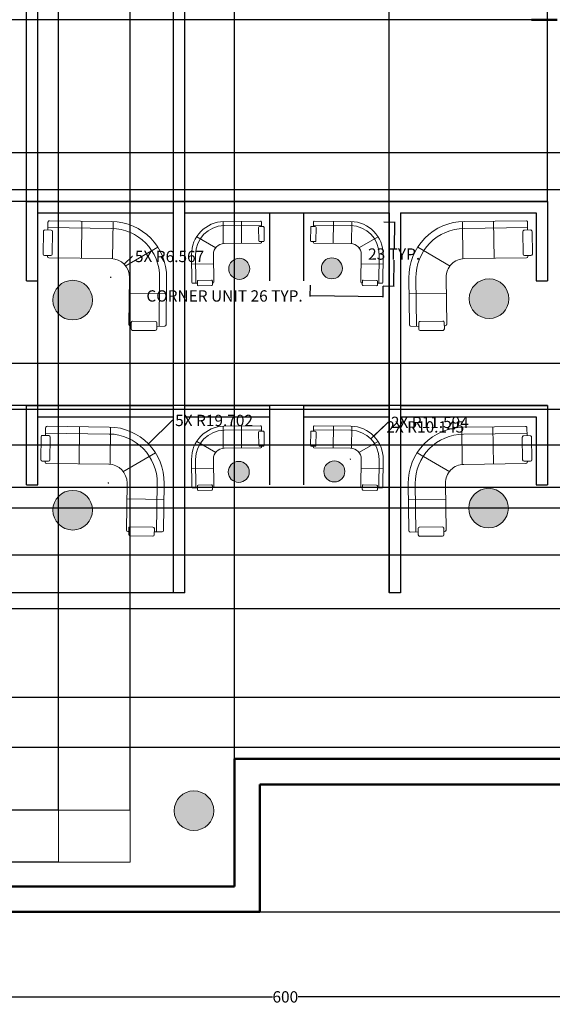
# Model space of a CAD drawing. Units: inches. Extents: x 1454 to 2136, y 626 to 1213.
# Tile 4 of 23: x 1699 to 1887, y 626 to 973. Entities that reach past the tile are written whole.
import ezdxf

# ---------------------------------------------------------------- set-up
doc = ezdxf.new("R2010")
doc.units = ezdxf.units.IN
doc.header["$MEASUREMENT"] = 0
for name, color, linetype, lineweight in [('A-ANNO-DIMS', 2, 'Continuous', 18), ('A-FURN', 9, 'Continuous', 18), ('A-FURN-PATT', 252, 'Continuous', 13), ('A-FURN-PNLS', 8, 'Continuous', 25), ('A-PLNT-PATT', 116, 'Continuous', 13), ('A-WALL', 7, 'Continuous', 50), ('leafs', 112, 'Continuous', 18), ('sofa', 4, 'Continuous', 18)]:
    doc.layers.add(name, color=color, linetype=linetype, lineweight=lineweight)
doc.styles.get("Standard").update_dxf_attribs({"font": 'arial.ttf'})
doc.dimstyles.get("Standard").update_dxf_attribs({"dimtxt": 4, "dimasz": 0.18, "dimexe": 0.18, "dimexo": 0.0625, "dimgap": 0.09, "dimtad": 0, "dimtih": 1, "dimtoh": 1, "dimdec": 0, "dimrnd": 6, "dimzin": 0, "dimdsep": 46, "dimlunit": 3, "dimtxsty": 'Standard', "dimcen": 0.09, "dimadec": 0, "dimazin": 0, "dimtfac": 1, "dimtdec": 0, "dimtofl": 0, "dimtmove": 0, "dimatfit": 3, "dimfxl": 1, "dimtolj": 1, "dimtzin": 0, "dimarcsym": 0})

# ---------------------------------------------------------------- blocks, each defined once
blk = doc.blocks.new('A$C42183DBB')
for p, q in [((0.166, 1.682), (0.518, 1.682)), ((0, 1.592), (0, 0.864)), ((0.022, 1.614), (0.144, 1.614)), ((0.108, 1.614), (0.108, 0.864)), ((0.144, 1.661), (0.144, 1.562)), ((0.166, 1.541), (0.518, 1.541)), ((0.54, 1.661), (0.54, 1.562)), ((0.54, 1.614), (0.554, 1.614)), ((0.576, 1.592), (0.576, 0.864)), ((0, 1.11), (0.576, 1.11)), ((0.643, 0.69), (0.142, 0.389)), ((0.84, 0.576), (0.84, 0)), ((0.864, 0.576), (1.826, 0.576)), ((1.322, 0.576), (1.322, 0)), ((1.775, 0.166), (1.775, 0.518)), ((1.895, 0.54), (1.797, 0.54)), ((1.848, 0.54), (1.848, 0.554)), ((1.917, 0.166), (1.917, 0.518)), ((0.864, 0.108), (1.848, 0.108)), ((1.895, 0.144), (1.797, 0.144)), ((1.848, 0.022), (1.848, 0.144)), ((0.864, 0), (1.826, 0))]:
    blk.add_line(p, q)
for centre, radius, start, end in [((0.166, 1.661), 0.0216, 90, 180), ((0.518, 1.661), 0.0216, 0, 90), ((0.022, 1.592), 0.0216, 90, 180), ((0.166, 1.562), 0.0216, 180, 270), ((0.518, 1.562), 0.0216, 270, 0), ((0.554, 1.592), 0.0216, 0, 90), ((0.864, 0.864), 0.864, 180, 270), ((0.864, 0.864), 0.756, 180, 270), ((0.864, 0.864), 0.288, 180, 270), ((1.797, 0.518), 0.0216, 90, 180), ((1.826, 0.554), 0.0216, 0, 90), ((1.895, 0.518), 0.0216, 0, 90), ((1.797, 0.166), 0.0216, 180, 270), ((1.895, 0.166), 0.0216, 270, 0), ((1.826, 0.022), 0.0216, 270, 0)]:
    blk.add_arc(centre, radius, start, end)
blk = doc.blocks.new('*D11')
at = {"layer": 'A-ANNO-DIMS', "color": 0, "lineweight": -2, "transparency": 16777216}
for p, q in [((1801.3, 879.55), (1801.25, 875.57)), ((1827.02, 879.24), (1826.97, 875.26)), ((1801.25, 875.75), (1801.07, 875.75)), ((1826.79, 875.44), (1801.43, 875.75))]:
    blk.add_line(p, q, dxfattribs=at)
at = {"layer": 'A-ANNO-DIMS', "color": 0, "transparency": 16777216}
for points in [[(1801.43, 875.78), (1801.43, 875.72), (1801.25, 875.75)], [(1826.79, 875.47), (1826.79, 875.41), (1826.97, 875.44)]]:
    blk.add_solid(points, dxfattribs=at)
at = {"layer": 'Defpoints', "color": 0, "transparency": 16777216}
for p in [(1801.3, 879.61), (1827.02, 879.3), (1801.25, 875.75)]:
    blk.add_point(p, dxfattribs=at)
at = {"layer": 'A-ANNO-DIMS', "color": 0, "transparency": 16777216, "insert": (1771.09, 875.75), "char_height": 4, "attachment_point": 5}
blk.add_mtext('\\A1;CORNER UNIT 26 TYP.', dxfattribs=at)
blk = doc.blocks.new('*D12')
at = {"layer": 'A-ANNO-DIMS', "color": 0, "lineweight": -2, "transparency": 16777216}
for p, q in [((1827.35, 901.87), (1831.33, 901.83)), ((1831.14, 901.65), (1831.04, 892.67)), ((1830.88, 879.43), (1830.98, 888.41)), ((1827.08, 879.3), (1831.05, 879.25))]:
    blk.add_line(p, q, dxfattribs=at)
at = {"layer": 'A-ANNO-DIMS', "color": 0, "transparency": 16777216}
for points in [[(1831.11, 901.65), (1831.17, 901.65), (1831.15, 901.83)], [(1830.85, 879.43), (1830.91, 879.43), (1830.87, 879.25)]]:
    blk.add_solid(points, dxfattribs=at)
at = {"layer": 'Defpoints', "color": 0, "transparency": 16777216}
for p in [(1827.29, 901.87), (1827.02, 879.3), (1830.87, 879.25)]:
    blk.add_point(p, dxfattribs=at)
at = {"layer": 'A-ANNO-DIMS', "color": 0, "transparency": 16777216, "insert": (1831.01, 890.54), "char_height": 4, "attachment_point": 5}
blk.add_mtext('\\A1;23 TYP.', dxfattribs=at)
blk = doc.blocks.new('*D27')
at = {"layer": 'A-ANNO-DIMS', "color": 0, "lineweight": -2, "transparency": 16777216}
for p, q in [((2092.56, 703.22), (2092.56, 628.1)), ((1492.56, 658.22), (1492.56, 628.1)), ((1492.74, 628.28), (1788.04, 628.28)), ((2092.38, 628.28), (1797.07, 628.28))]:
    blk.add_line(p, q, dxfattribs=at)
at = {"layer": 'A-ANNO-DIMS', "color": 0, "transparency": 16777216}
for points in [[(1492.74, 628.31), (1492.74, 628.25), (1492.56, 628.28)], [(2092.38, 628.31), (2092.38, 628.25), (2092.56, 628.28)]]:
    blk.add_solid(points, dxfattribs=at)
at = {"layer": 'Defpoints', "color": 0, "transparency": 16777216}
for p in [(2092.56, 703.28), (1492.56, 658.28), (2092.56, 628.28)]:
    blk.add_point(p, dxfattribs=at)
at = {"layer": 'A-ANNO-DIMS', "color": 0, "transparency": 16777216, "insert": (1792.56, 628.28), "char_height": 4, "attachment_point": 5}
blk.add_mtext('\\A1;600', dxfattribs=at)
blk = doc.blocks.new('*D37')
at = {"layer": 'A-ANNO-DIMS', "color": 0, "lineweight": -2, "transparency": 16777216}
for p, q in [((1774.56, 712.34), (1774.56, 1210.46)), ((1774.74, 1210.28), (1846.74, 1210.28)), ((1927.38, 1210.28), (1855.38, 1210.28)), ((1927.56, 712.34), (1927.56, 1210.46))]:
    blk.add_line(p, q, dxfattribs=at)
at = {"layer": 'A-ANNO-DIMS', "color": 0, "transparency": 16777216}
for points in [[(1774.74, 1210.31), (1774.74, 1210.25), (1774.56, 1210.28)], [(1927.38, 1210.31), (1927.38, 1210.25), (1927.56, 1210.28)]]:
    blk.add_solid(points, dxfattribs=at)
at = {"layer": 'Defpoints', "color": 0, "transparency": 16777216}
for p in [(1927.56, 1210.28), (1774.56, 712.28), (1927.56, 712.28)]:
    blk.add_point(p, dxfattribs=at)
at = {"layer": 'A-ANNO-DIMS', "color": 0, "transparency": 16777216, "insert": (1851.06, 1210.28), "char_height": 4, "attachment_point": 5}
blk.add_mtext('\\A1;153', dxfattribs=at)
blk = doc.blocks.new('*D38')
at = {"layer": 'A-ANNO-DIMS', "color": 0, "lineweight": -2, "transparency": 16777216}
for p, q in [((1783.62, 703.28), (2122.74, 703.28)), ((2122.56, 703.1), (2122.56, 682.91)), ((2122.56, 658.46), (2122.56, 678.66)), ((1783.62, 658.28), (2122.74, 658.28))]:
    blk.add_line(p, q, dxfattribs=at)
at = {"layer": 'A-ANNO-DIMS', "color": 0, "transparency": 16777216}
for points in [[(2122.53, 703.1), (2122.59, 703.1), (2122.56, 703.28)], [(2122.53, 658.46), (2122.59, 658.46), (2122.56, 658.28)]]:
    blk.add_solid(points, dxfattribs=at)
at = {"layer": 'Defpoints', "color": 0, "transparency": 16777216}
for p in [(1783.56, 703.28), (2122.56, 703.28), (1783.56, 658.28)]:
    blk.add_point(p, dxfattribs=at)
at = {"layer": 'A-ANNO-DIMS', "color": 0, "transparency": 16777216, "insert": (2122.56, 680.78), "char_height": 4, "attachment_point": 5}
blk.add_mtext('\\A1;45', dxfattribs=at)
blk = doc.blocks.new('*D44')
at = {"layer": 'A-ANNO-DIMS', "color": 0, "lineweight": -2, "transparency": 16777216}
for p, q in [((1701.08, 909.11), (1701.08, 1210.46)), ((1701.26, 1210.28), (1784.96, 1210.28)), ((1885.07, 1210.28), (1801.37, 1210.28)), ((1885.25, 909.11), (1885.25, 1210.46))]:
    blk.add_line(p, q, dxfattribs=at)
at = {"layer": 'A-ANNO-DIMS', "color": 0, "transparency": 16777216}
for points in [[(1701.26, 1210.31), (1701.26, 1210.25), (1701.08, 1210.28)], [(1885.07, 1210.31), (1885.07, 1210.25), (1885.25, 1210.28)]]:
    blk.add_solid(points, dxfattribs=at)
at = {"layer": 'Defpoints', "color": 0, "transparency": 16777216}
for p in [(1885.25, 1210.28), (1701.08, 909.05), (1885.25, 909.05)]:
    blk.add_point(p, dxfattribs=at)
at = {"layer": 'A-ANNO-DIMS', "color": 0, "transparency": 16777216, "insert": (1793.16, 1210.28), "char_height": 4, "attachment_point": 5}
blk.add_mtext('\\A1;184.17', dxfattribs=at)
blk = doc.blocks.new('*D45')
at = {"layer": 'A-ANNO-DIMS', "color": 0, "lineweight": -2, "transparency": 16777216}
for p, q in [((1654.56, 913.34), (1654.56, 1210.46)), ((1654.74, 1210.28), (1670.92, 1210.28)), ((1700.9, 1210.28), (1684.72, 1210.28)), ((1701.08, 909.11), (1701.08, 1210.46))]:
    blk.add_line(p, q, dxfattribs=at)
at = {"layer": 'A-ANNO-DIMS', "color": 0, "transparency": 16777216}
for points in [[(1654.74, 1210.31), (1654.74, 1210.25), (1654.56, 1210.28)], [(1700.9, 1210.31), (1700.9, 1210.25), (1701.08, 1210.28)]]:
    blk.add_solid(points, dxfattribs=at)
at = {"layer": 'Defpoints', "color": 0, "transparency": 16777216}
for p in [(1701.08, 1210.28), (1654.56, 913.28), (1701.08, 909.05)]:
    blk.add_point(p, dxfattribs=at)
at = {"layer": 'A-ANNO-DIMS', "color": 0, "transparency": 16777216, "insert": (1677.82, 1210.28), "char_height": 4, "attachment_point": 5}
blk.add_mtext('\\A1;46.52', dxfattribs=at)
blk = doc.blocks.new('*D46')
at = {"layer": 'A-ANNO-DIMS', "color": 0, "lineweight": -2, "transparency": 16777216}
for p, q in [((1701.01, 909.05), (1462.37, 909.05)), ((1462.55, 908.87), (1462.55, 842.13)), ((1462.55, 771.13), (1462.55, 837.86)), ((1753.01, 770.95), (1462.37, 770.95))]:
    blk.add_line(p, q, dxfattribs=at)
at = {"layer": 'A-ANNO-DIMS', "color": 0, "transparency": 16777216}
for points in [[(1462.52, 908.87), (1462.58, 908.87), (1462.55, 909.05)], [(1462.52, 771.13), (1462.58, 771.13), (1462.55, 770.95)]]:
    blk.add_solid(points, dxfattribs=at)
at = {"layer": 'Defpoints', "color": 0, "transparency": 16777216}
for p in [(1701.08, 909.05), (1462.55, 770.95), (1753.08, 770.95)]:
    blk.add_point(p, dxfattribs=at)
at = {"layer": 'A-ANNO-DIMS', "color": 0, "transparency": 16777216, "insert": (1462.55, 840), "char_height": 4, "attachment_point": 5}
blk.add_mtext('\\A1;138.1', dxfattribs=at)
blk = doc.blocks.new('*D47')
at = {"layer": 'A-ANNO-DIMS', "color": 0, "lineweight": -2, "transparency": 16777216}
for p, q in [((1885.25, 909.11), (1885.25, 1210.46)), ((1885.43, 1210.28), (1899.87, 1210.28)), ((1927.38, 1210.28), (1912.94, 1210.28)), ((1927.56, 910.34), (1927.56, 1210.46))]:
    blk.add_line(p, q, dxfattribs=at)
at = {"layer": 'A-ANNO-DIMS', "color": 0, "transparency": 16777216}
for points in [[(1885.43, 1210.31), (1885.43, 1210.25), (1885.25, 1210.28)], [(1927.38, 1210.31), (1927.38, 1210.25), (1927.56, 1210.28)]]:
    blk.add_solid(points, dxfattribs=at)
at = {"layer": 'Defpoints', "color": 0, "transparency": 16777216}
for p in [(1885.25, 1210.28), (1885.25, 909.05), (1927.56, 910.28)]:
    blk.add_point(p, dxfattribs=at)
at = {"layer": 'A-ANNO-DIMS', "color": 0, "transparency": 16777216, "insert": (1906.4, 1210.28), "char_height": 4, "attachment_point": 5}
blk.add_mtext('\\A1;42.31', dxfattribs=at)
blk = doc.blocks.new('*D48')
at = {"layer": 'A-ANNO-DIMS', "color": 0, "lineweight": -2, "transparency": 16777216}
for p, q in [((1879.49, 973.28), (1462.37, 973.28)), ((1462.55, 973.1), (1462.55, 943.3)), ((1462.55, 909.23), (1462.55, 939.03)), ((1885.19, 909.05), (1462.37, 909.05))]:
    blk.add_line(p, q, dxfattribs=at)
at = {"layer": 'A-ANNO-DIMS', "color": 0, "transparency": 16777216}
for points in [[(1462.52, 973.1), (1462.58, 973.1), (1462.55, 973.28)], [(1462.52, 909.23), (1462.58, 909.23), (1462.55, 909.05)]]:
    blk.add_solid(points, dxfattribs=at)
at = {"layer": 'Defpoints', "color": 0, "transparency": 16777216}
for p in [(1879.56, 973.28), (1462.55, 909.05), (1885.25, 909.05)]:
    blk.add_point(p, dxfattribs=at)
at = {"layer": 'A-ANNO-DIMS', "color": 0, "transparency": 16777216, "insert": (1462.55, 941.17), "char_height": 4, "attachment_point": 5}
blk.add_mtext('\\A1;64.23', dxfattribs=at)
blk = doc.blocks.new('*D52')
at = {"layer": 'A-ANNO-DIMS', "color": 0, "lineweight": -2, "transparency": 16777216}
for p, q in [((1927.57, 800.77), (1462.37, 800.77)), ((1462.55, 800.59), (1462.55, 794.66)), ((1462.55, 784.46), (1462.55, 790.4)), ((1927.49, 784.28), (1462.37, 784.28))]:
    blk.add_line(p, q, dxfattribs=at)
at = {"layer": 'A-ANNO-DIMS', "color": 0, "transparency": 16777216}
for points in [[(1462.52, 800.59), (1462.58, 800.59), (1462.55, 800.77)], [(1462.52, 784.46), (1462.58, 784.46), (1462.55, 784.28)]]:
    blk.add_solid(points, dxfattribs=at)
at = {"layer": 'Defpoints', "color": 0, "transparency": 16777216}
for p in [(1462.55, 800.77), (1927.64, 800.77), (1927.56, 784.28)]:
    blk.add_point(p, dxfattribs=at)
at = {"layer": 'A-ANNO-DIMS', "color": 0, "transparency": 16777216, "insert": (1462.55, 792.53), "char_height": 4, "attachment_point": 5}
blk.add_mtext('\\A1;16.49', dxfattribs=at)
blk = doc.blocks.new('*D53')
at = {"layer": 'A-ANNO-DIMS', "color": 0, "lineweight": -2, "transparency": 16777216}
for p, q in [((1927.57, 851.9), (1462.37, 851.9)), ((1462.55, 851.72), (1462.55, 845.89)), ((1462.55, 835.79), (1462.55, 841.63)), ((1927.57, 835.61), (1462.37, 835.61))]:
    blk.add_line(p, q, dxfattribs=at)
at = {"layer": 'A-ANNO-DIMS', "color": 0, "transparency": 16777216}
for points in [[(1462.52, 851.72), (1462.58, 851.72), (1462.55, 851.9)], [(1462.52, 835.79), (1462.58, 835.79), (1462.55, 835.61)]]:
    blk.add_solid(points, dxfattribs=at)
at = {"layer": 'Defpoints', "color": 0, "transparency": 16777216}
for p in [(1462.55, 851.9), (1927.64, 851.9), (1927.64, 835.61)]:
    blk.add_point(p, dxfattribs=at)
at = {"layer": 'A-ANNO-DIMS', "color": 0, "transparency": 16777216, "insert": (1462.55, 843.76), "char_height": 4, "attachment_point": 5}
blk.add_mtext('\\A1;16.29', dxfattribs=at)
blk = doc.blocks.new('*D57')
at = {"layer": 'A-ANNO-DIMS', "color": 0, "lineweight": -2, "transparency": 16777216}
for p, q in [((1654.43, 823.23), (2122.74, 823.23)), ((2122.56, 823.05), (2122.56, 817.89)), ((2122.56, 808.46), (2122.56, 813.62)), ((1654.62, 808.28), (2122.74, 808.28))]:
    blk.add_line(p, q, dxfattribs=at)
at = {"layer": 'A-ANNO-DIMS', "color": 0, "transparency": 16777216}
for points in [[(2122.53, 823.05), (2122.59, 823.05), (2122.56, 823.23)], [(2122.53, 808.46), (2122.59, 808.46), (2122.56, 808.28)]]:
    blk.add_solid(points, dxfattribs=at)
at = {"layer": 'Defpoints', "color": 0, "transparency": 16777216}
for p in [(1654.37, 823.23), (2122.56, 823.23), (1654.56, 808.28)]:
    blk.add_point(p, dxfattribs=at)
at = {"layer": 'A-ANNO-DIMS', "color": 0, "transparency": 16777216, "insert": (2122.56, 815.75), "char_height": 4, "attachment_point": 5}
blk.add_mtext('\\A1;14.944', dxfattribs=at)
blk = doc.blocks.new('*D58')
at = {"layer": 'A-ANNO-DIMS', "color": 0, "lineweight": -2, "transparency": 16777216}
for p, q in [((1654.43, 926.36), (2122.74, 926.36)), ((2122.56, 926.18), (2122.56, 921.96)), ((2122.56, 913.46), (2122.56, 917.69)), ((1654.62, 913.28), (2122.74, 913.28))]:
    blk.add_line(p, q, dxfattribs=at)
at = {"layer": 'A-ANNO-DIMS', "color": 0, "transparency": 16777216}
for points in [[(2122.53, 926.18), (2122.59, 926.18), (2122.56, 926.36)], [(2122.53, 913.46), (2122.59, 913.46), (2122.56, 913.28)]]:
    blk.add_solid(points, dxfattribs=at)
at = {"layer": 'Defpoints', "color": 0, "transparency": 16777216}
for p in [(1654.37, 926.36), (2122.56, 926.36), (1654.56, 913.28)]:
    blk.add_point(p, dxfattribs=at)
at = {"layer": 'A-ANNO-DIMS', "color": 0, "transparency": 16777216, "insert": (2122.56, 919.82), "char_height": 4, "attachment_point": 5}
blk.add_mtext('\\A1;13.082', dxfattribs=at)
blk = doc.blocks.new('*D64')
at = {"layer": 'A-ANNO-DIMS', "color": 0, "lineweight": -2, "transparency": 16777216}
for p, q in [((2000.57, 733.92), (1462.37, 733.92)), ((1462.55, 733.74), (1462.55, 727.25)), ((1462.55, 716.5), (1462.55, 722.99)), ((2000.57, 716.32), (1462.37, 716.32))]:
    blk.add_line(p, q, dxfattribs=at)
at = {"layer": 'A-ANNO-DIMS', "color": 0, "transparency": 16777216}
for points in [[(1462.52, 733.74), (1462.58, 733.74), (1462.55, 733.92)], [(1462.52, 716.5), (1462.58, 716.5), (1462.55, 716.32)]]:
    blk.add_solid(points, dxfattribs=at)
at = {"layer": 'Defpoints', "color": 0, "transparency": 16777216}
for p in [(1462.55, 733.92), (2000.63, 733.92), (2000.63, 716.32)]:
    blk.add_point(p, dxfattribs=at)
at = {"layer": 'A-ANNO-DIMS', "color": 0, "transparency": 16777216, "insert": (1462.55, 725.12), "char_height": 4, "attachment_point": 5}
blk.add_mtext('\\A1;17.604', dxfattribs=at)
blk = doc.blocks.new('*D65')
at = {"layer": 'A-ANNO-DIMS', "color": 0, "lineweight": -2, "transparency": 16777216}
for p, q in [((1885.19, 909.05), (1462.37, 909.05)), ((1462.55, 908.87), (1462.55, 875.15)), ((1462.55, 837.23), (1462.55, 870.95)), ((1885.19, 837.05), (1462.37, 837.05))]:
    blk.add_line(p, q, dxfattribs=at)
at = {"layer": 'A-ANNO-DIMS', "color": 0, "transparency": 16777216}
for points in [[(1462.52, 908.87), (1462.58, 908.87), (1462.55, 909.05)], [(1462.52, 837.23), (1462.58, 837.23), (1462.55, 837.05)]]:
    blk.add_solid(points, dxfattribs=at)
at = {"layer": 'Defpoints', "color": 0, "transparency": 16777216}
for p in [(1885.25, 909.05), (1462.55, 837.05), (1885.25, 837.05)]:
    blk.add_point(p, dxfattribs=at)
at = {"layer": 'A-ANNO-DIMS', "color": 0, "transparency": 16777216, "insert": (1462.55, 873.05), "char_height": 4, "attachment_point": 5}
blk.add_mtext('\\A1;72', dxfattribs=at)
blk = doc.blocks.new('*D66')
at = {"layer": 'A-ANNO-DIMS', "color": 0, "lineweight": -2, "transparency": 16777216}
for p, q in [((1757.08, 771.01), (1757.08, 1210.46)), ((1757.26, 1210.28), (1786.34, 1210.28)), ((1829.07, 1210.28), (1799.99, 1210.28)), ((1829.25, 771.01), (1829.25, 1210.46))]:
    blk.add_line(p, q, dxfattribs=at)
at = {"layer": 'A-ANNO-DIMS', "color": 0, "transparency": 16777216}
for points in [[(1757.26, 1210.31), (1757.26, 1210.25), (1757.08, 1210.28)], [(1829.07, 1210.31), (1829.07, 1210.25), (1829.25, 1210.28)]]:
    blk.add_solid(points, dxfattribs=at)
at = {"layer": 'Defpoints', "color": 0, "transparency": 16777216}
for p in [(1829.25, 1210.28), (1757.08, 770.95), (1829.25, 770.95)]:
    blk.add_point(p, dxfattribs=at)
at = {"layer": 'A-ANNO-DIMS', "color": 0, "transparency": 16777216, "insert": (1793.16, 1210.28), "char_height": 4, "attachment_point": 5}
blk.add_mtext('\\A1;72.17', dxfattribs=at)
blk = doc.blocks.new('*D71')
at = {"layer": 'A-ANNO-DIMS', "color": 0, "lineweight": -2, "transparency": 16777216}
for p, q in [((1712.39, 694.26), (1712.39, 1210.46)), ((1712.57, 1210.28), (1718.61, 1210.28)), ((1737.62, 1210.28), (1731.58, 1210.28)), ((1737.8, 694.26), (1737.8, 1210.46))]:
    blk.add_line(p, q, dxfattribs=at)
at = {"layer": 'A-ANNO-DIMS', "color": 0, "transparency": 16777216}
for points in [[(1712.57, 1210.31), (1712.57, 1210.25), (1712.39, 1210.28)], [(1737.62, 1210.31), (1737.62, 1210.25), (1737.8, 1210.28)]]:
    blk.add_solid(points, dxfattribs=at)
at = {"layer": 'Defpoints', "color": 0, "transparency": 16777216}
for p in [(1737.8, 1210.28), (1712.39, 694.2), (1737.8, 694.2)]:
    blk.add_point(p, dxfattribs=at)
at = {"layer": 'A-ANNO-DIMS', "color": 0, "transparency": 16777216, "insert": (1725.09, 1210.28), "char_height": 4, "attachment_point": 5}
blk.add_mtext('\\A1;25.41', dxfattribs=at)
blk = doc.blocks.new('*D72')
at = {"layer": 'A-ANNO-DIMS', "color": 0, "lineweight": -2, "transparency": 16777216}
for p, q in [((1712.33, 694.2), (1462.37, 694.2)), ((1462.55, 694.02), (1462.55, 687.17)), ((1462.55, 676.04), (1462.55, 682.9)), ((1712.33, 675.86), (1462.37, 675.86))]:
    blk.add_line(p, q, dxfattribs=at)
at = {"layer": 'A-ANNO-DIMS', "color": 0, "transparency": 16777216}
for points in [[(1462.52, 694.02), (1462.58, 694.02), (1462.55, 694.2)], [(1462.52, 676.04), (1462.58, 676.04), (1462.55, 675.86)]]:
    blk.add_solid(points, dxfattribs=at)
at = {"layer": 'Defpoints', "color": 0, "transparency": 16777216}
for p in [(1462.55, 694.2), (1712.39, 694.2), (1712.39, 675.86)]:
    blk.add_point(p, dxfattribs=at)
at = {"layer": 'A-ANNO-DIMS', "color": 0, "transparency": 16777216, "insert": (1462.55, 685.03), "char_height": 4, "attachment_point": 5}
blk.add_mtext('\\A1;18.338', dxfattribs=at)
blk = doc.blocks.new('*D77')
at = {"layer": 'A-ANNO-DIMS', "color": 0, "lineweight": -2, "transparency": 16777216}
for p, q in [((1753.08, 771.01), (1753.08, 1210.46)), ((1753.26, 1210.28), (1753.6, 1210.28)), ((1756.9, 1210.28), (1756.55, 1210.28)), ((1757.08, 771.01), (1757.08, 1210.46))]:
    blk.add_line(p, q, dxfattribs=at)
at = {"layer": 'A-ANNO-DIMS', "color": 0, "transparency": 16777216}
for points in [[(1753.26, 1210.31), (1753.26, 1210.25), (1753.08, 1210.28)], [(1756.9, 1210.31), (1756.9, 1210.25), (1757.08, 1210.28)]]:
    blk.add_solid(points, dxfattribs=at)
at = {"layer": 'Defpoints', "color": 0, "transparency": 16777216}
for p in [(1757.08, 1210.28), (1753.08, 770.95), (1757.08, 770.95)]:
    blk.add_point(p, dxfattribs=at)
at = {"layer": 'A-ANNO-DIMS', "color": 0, "transparency": 16777216, "insert": (1755.08, 1210.28), "char_height": 4, "attachment_point": 5}
blk.add_mtext('\\A1;4', dxfattribs=at)
blk = doc.blocks.new('*D78')
at = {"layer": 'A-ANNO-DIMS', "color": 0, "lineweight": -2, "transparency": 16777216}
for p, q in [((1705.08, 833.11), (1705.08, 1210.46)), ((1705.26, 1210.28), (1726.04, 1210.28)), ((1752.9, 1210.28), (1732.12, 1210.28)), ((1753.08, 833.11), (1753.08, 1210.46))]:
    blk.add_line(p, q, dxfattribs=at)
at = {"layer": 'A-ANNO-DIMS', "color": 0, "transparency": 16777216}
for points in [[(1705.26, 1210.31), (1705.26, 1210.25), (1705.08, 1210.28)], [(1752.9, 1210.31), (1752.9, 1210.25), (1753.08, 1210.28)]]:
    blk.add_solid(points, dxfattribs=at)
at = {"layer": 'Defpoints', "color": 0, "transparency": 16777216}
for p in [(1753.08, 1210.28), (1705.08, 833.05), (1753.08, 833.05)]:
    blk.add_point(p, dxfattribs=at)
at = {"layer": 'A-ANNO-DIMS', "color": 0, "transparency": 16777216, "insert": (1729.08, 1210.28), "char_height": 4, "attachment_point": 5}
blk.add_mtext('\\A1;48', dxfattribs=at)
blk = doc.blocks.new('*D87')
at = {"layer": 'A-ANNO-DIMS', "color": 0, "lineweight": -2, "transparency": 16777216}
for p, q in [((2076.36, 765.24), (1462.37, 765.24)), ((1462.55, 765.06), (1462.55, 751.71)), ((1462.55, 734.1), (1462.55, 747.45)), ((2081.97, 733.92), (1462.37, 733.92))]:
    blk.add_line(p, q, dxfattribs=at)
at = {"layer": 'A-ANNO-DIMS', "color": 0, "transparency": 16777216}
for points in [[(1462.52, 765.06), (1462.58, 765.06), (1462.55, 765.24)], [(1462.52, 734.1), (1462.58, 734.1), (1462.55, 733.92)]]:
    blk.add_solid(points, dxfattribs=at)
at = {"layer": 'Defpoints', "color": 0, "transparency": 16777216}
for p in [(1462.55, 765.24), (2076.42, 765.24), (2082.04, 733.92)]:
    blk.add_point(p, dxfattribs=at)
at = {"layer": 'A-ANNO-DIMS', "color": 0, "transparency": 16777216, "insert": (1462.55, 749.58), "char_height": 4, "attachment_point": 5}
blk.add_mtext('\\A1;31.32', dxfattribs=at)
blk = doc.blocks.new('*D99')
at = {"layer": 'A-ANNO-DIMS', "color": 0, "lineweight": -2, "transparency": 16777216}
for p, q in [((1752.62, 831.79), (1744.29, 823.66)), ((1752.8, 831.79), (1752.62, 831.79)), ((1729.98, 809.77), (1730.16, 809.77)), ((1730.07, 809.68), (1730.07, 809.86))]:
    blk.add_line(p, q, dxfattribs=at)
at = {"layer": 'A-ANNO-DIMS', "color": 0, "transparency": 16777216}
blk.add_solid([(1744.27, 823.68), (1744.32, 823.64), (1744.17, 823.53)], dxfattribs=at)
at = {"layer": 'Defpoints', "color": 0, "transparency": 16777216}
for p in [(1744.17, 823.53), (1730.07, 809.77)]:
    blk.add_point(p, dxfattribs=at)
at = {"layer": 'A-ANNO-DIMS', "color": 0, "transparency": 16777216, "insert": (1767.39, 831.79), "char_height": 4, "attachment_point": 5}
blk.add_mtext('\\A1;5X R19.702', dxfattribs=at)
blk = doc.blocks.new('*D101')
at = {"layer": 'A-ANNO-DIMS', "color": 0, "lineweight": -2, "transparency": 16777216}
for p, q in [((1828.83, 831.12), (1823.98, 826.38)), ((1829.01, 831.12), (1828.83, 831.12)), ((1815.46, 818.16), (1815.64, 818.16)), ((1815.55, 818.07), (1815.55, 818.25))]:
    blk.add_line(p, q, dxfattribs=at)
at = {"layer": 'A-ANNO-DIMS', "color": 0, "transparency": 16777216}
blk.add_solid([(1823.96, 826.41), (1824, 826.36), (1823.85, 826.26)], dxfattribs=at)
at = {"layer": 'Defpoints', "color": 0, "transparency": 16777216}
for p in [(1823.85, 826.26), (1815.55, 818.16)]:
    blk.add_point(p, dxfattribs=at)
at = {"layer": 'A-ANNO-DIMS', "color": 0, "transparency": 16777216, "insert": (1843.64, 831.12), "char_height": 4, "attachment_point": 5}
blk.add_mtext('\\A1;2X R11.594', dxfattribs=at)
blk = doc.blocks.new('*D102')
at = {"layer": 'A-ANNO-DIMS', "color": 0, "lineweight": -2, "transparency": 16777216}
for p, q in [((1827.17, 829.5), (1822.94, 825.37)), ((1827.35, 829.5), (1827.17, 829.5)), ((1815.46, 818.16), (1815.64, 818.16)), ((1815.55, 818.07), (1815.55, 818.25))]:
    blk.add_line(p, q, dxfattribs=at)
at = {"layer": 'A-ANNO-DIMS', "color": 0, "transparency": 16777216}
blk.add_solid([(1822.92, 825.39), (1822.96, 825.35), (1822.81, 825.25)], dxfattribs=at)
at = {"layer": 'Defpoints', "color": 0, "transparency": 16777216}
for p in [(1822.81, 825.25), (1815.55, 818.16)]:
    blk.add_point(p, dxfattribs=at)
at = {"layer": 'A-ANNO-DIMS', "color": 0, "transparency": 16777216, "insert": (1842, 829.5), "char_height": 4, "attachment_point": 5}
blk.add_mtext('\\A1;2X R10.145', dxfattribs=at)
blk = doc.blocks.new('*D103')
at = {"layer": 'A-ANNO-DIMS', "color": 0, "lineweight": -2, "transparency": 16777216}
for p, q in [((1738.43, 889.69), (1735.74, 887.07)), ((1738.61, 889.69), (1738.43, 889.69)), ((1730.82, 882.35), (1731, 882.35)), ((1730.91, 882.26), (1730.91, 882.44))]:
    blk.add_line(p, q, dxfattribs=at)
at = {"layer": 'A-ANNO-DIMS', "color": 0, "transparency": 16777216}
blk.add_solid([(1735.72, 887.09), (1735.76, 887.04), (1735.61, 886.94)], dxfattribs=at)
at = {"layer": 'Defpoints', "color": 0, "transparency": 16777216}
for p in [(1735.61, 886.94), (1730.91, 882.35)]:
    blk.add_point(p, dxfattribs=at)
at = {"layer": 'A-ANNO-DIMS', "color": 0, "transparency": 16777216, "insert": (1751.66, 889.69), "char_height": 4, "attachment_point": 5}
blk.add_mtext('\\A1;5X R6.567', dxfattribs=at)

msp = doc.modelspace()

# ---------------------------------------------------------------- hatches: boundary and pattern name
at = {"layer": 'A-FURN-PATT'}
h = msp.add_hatch(dxfattribs=at)
h.set_pattern_fill('ESCHER', color=256)
h.paths.add_polyline_path([(1511.3761, 923.7174, 1), (1525.379, 923.7174, 1)])
h.paths.add_polyline_path([(1525.379, 816.0542, 1), (1511.3761, 816.0542, 1)])
h.paths.add_polyline_path([(1525.379, 712.7345, 1), (1511.3761, 712.7345, 1)])
h.paths.add_polyline_path([(2070.5057, 794.3402, 1), (2056.5027, 794.3402, 1)])
h.paths.add_polyline_path([(2005.868, 1014.5578, 1), (1991.8651, 1014.5578, 1)])
h.paths.add_polyline_path([(1994.0647, 1066.7584, 1), (2008.0677, 1066.7584, 1)])
h.paths.add_polyline_path([(1919.5492, 1065.3848, 1), (1933.5521, 1065.3848, 1)])
h.paths.add_polyline_path([(1936.8517, 1013.7336, 1), (1922.8488, 1013.7336, 1)])
h.paths.add_polyline_path([(1824.6062, 1109.1557, 1), (1838.6091, 1109.1557, 1)])
h = msp.add_hatch(dxfattribs=at)
h.set_pattern_fill('ESCHER', color=256)
h.paths.add_polyline_path([(1724.4407, 800.1118, 1), (1710.4377, 800.1118, 1)])
h.paths.add_polyline_path([(1779.8203, 813.6134, 1), (1772.4003, 813.6134, 1)])
h.paths.add_polyline_path([(1813.5888, 813.7882, 1), (1806.1687, 813.7882, 1)])
h.paths.add_polyline_path([(1871.3775, 800.8359, 1), (1857.3745, 800.8359, 1)])
h.paths.add_polyline_path([(1871.5488, 874.7673, 1), (1857.5458, 874.7673, 1)])
h.paths.add_polyline_path([(1812.7167, 885.4937, 1), (1805.2967, 885.4937, 1)])
h.paths.add_polyline_path([(1772.5781, 885.3189, 1), (1779.9981, 885.3189, 1)])
h.paths.add_polyline_path([(1724.4407, 874.2784, 1), (1710.4377, 874.2784, 1)])
at = {"layer": 'A-PLNT-PATT'}
h = msp.add_hatch(dxfattribs=at)
h.set_pattern_fill('ESCHER', color=256)
h.paths.add_polyline_path([(1767.2815, 694.0009, 1), (1753.2786, 694.0009, 1)])
h.paths.add_polyline_path([(1578.6873, 1043.8029, 1), (1564.6844, 1043.8029, 1)])

# ---------------------------------------------------------------- linework, layer by layer
at = {"layer": 'A-FURN'}
msp.add_lwpolyline([(1712.3887, 694.2005), (1737.8001, 694.2005), (1737.8001, 675.8628), (1712.3887, 675.8628)], close=True, dxfattribs=at)
for centre, radius in [((1776.2881, 885.3189), 3.71), ((1809.0067, 885.4937), 3.71), ((1717.4392, 874.2784), 7.0015), ((1864.5473, 874.7673), 7.0015), ((1776.1103, 813.6134), 3.71), ((1809.8788, 813.7882), 3.71), ((1717.4392, 800.1118), 7.0015), ((1864.376, 800.8359), 7.0015)]:
    msp.add_circle(centre, radius, dxfattribs=at)
at = {"layer": 'A-FURN-PNLS'}
for p, q in [((1701.0763, 909.0476), (1885.2497, 909.0476)), ((1701.0763, 881.0476), (1701.0763, 909.0476)), ((1885.2497, 909.0476), (1885.2497, 881.0476)), ((1705.0763, 905.0476), (1753.0763, 905.0476)), ((1705.0763, 881.0476), (1705.0763, 905.0476)), ((1753.0763, 837.0476), (1753.0763, 905.0476)), ((1757.0763, 837.0476), (1757.0763, 905.0476)), ((1757.0763, 905.0476), (1829.2497, 905.0476)), ((1787.0763, 881.0476), (1787.0763, 905.0476)), ((1799.0763, 881.0476), (1799.0763, 905.0476)), ((1829.2497, 905.0476), (1829.2497, 770.9473)), ((1833.2497, 905.0476), (1833.2497, 770.9473)), ((1833.2497, 905.0476), (1881.2497, 905.0476)), ((1881.2497, 905.0476), (1881.2497, 881.0476)), ((1701.0763, 881.0476), (1705.0763, 881.0476)), ((1881.2497, 881.0476), (1885.2497, 881.0476)), ((1701.0763, 809.0476), (1701.0763, 837.0476)), ((1701.0763, 837.0476), (1753.0763, 837.0476)), ((1757.0763, 837.0476), (1787.0763, 837.0476)), ((1787.0763, 809.0476), (1787.0763, 837.0476)), ((1799.0763, 809.0476), (1799.0763, 837.0476)), ((1799.0763, 837.0476), (1829.2497, 837.0476)), ((1833.2497, 837.0476), (1885.2497, 837.0476)), ((1885.2497, 837.0476), (1885.2497, 809.0476)), ((1705.0763, 809.0476), (1705.0763, 833.0476)), ((1705.0763, 833.0476), (1753.0763, 833.0476)), ((1753.0763, 770.9473), (1753.0763, 833.0476)), ((1757.0763, 770.9473), (1757.0763, 833.0476)), ((1757.0763, 833.0476), (1787.0763, 833.0476)), ((1799.0763, 833.0476), (1829.2497, 833.0476)), ((1833.2497, 833.0476), (1881.2497, 833.0476)), ((1881.2497, 833.0476), (1881.2497, 809.0476)), ((1701.0763, 809.0476), (1705.0763, 809.0476)), ((1881.2497, 809.0476), (1885.2497, 809.0476)), ((1757.0763, 770.9473), (1753.0763, 770.9473)), ((1833.2497, 770.9473), (1829.2497, 770.9473))]:
    msp.add_line(p, q, dxfattribs=at)
at = {"layer": 'A-WALL'}
for p, q in [((1888.5563, 973.2825), (1879.5563, 973.2825)), ((2083.5563, 712.2825), (1774.5563, 712.2825)), ((1774.5563, 712.2825), (1774.5563, 667.2825)), ((2092.5563, 703.2825), (1783.5563, 703.2825)), ((1783.5563, 703.2825), (1783.5563, 658.2825)), ((1774.5563, 667.2825), (1501.5563, 667.2825)), ((1783.5563, 658.2825), (1501.5563, 658.2825))]:
    msp.add_line(p, q, dxfattribs=at)
at = {"layer": 'leafs'}
msp.add_circle((1760.2801, 694.0009), 7.0015, dxfattribs=at)

# ---------------------------------------------------------------- block references
at = {"layer": 'sofa'}
for p, xscale, yscale, zscale, rotation in [((1750.8496, 901.8162), 22.80350778510874, 22.80350778510874, 22.80350778510874, 179.3111670300788), ((1759.2908, 901.8744), -13.41944498843718, 13.41944498843718, 13.41944498843718, 180.6888329699211), ((1827.2877, 901.8744), 13.41944498843718, 13.41944498843718, 13.41944498843718, 179.3111670300788), ((1836.0036, 901.8162), -22.80350778510874, 22.80350778510874, 22.80350778510874, 180.6888329699211), ((1750.0049, 829.2323), 22.80350778510874, 22.80350778510874, 22.80350778510874, 179.3111670300788), ((1759.2908, 829.6139), -13.41944498843718, 13.41944498843718, 13.41944498843718, 180.6888329699211), ((1827.2877, 829.6139), 13.41944498843718, 13.41944498843718, 13.41944498843718, 179.3111670300788), ((1835.7851, 829.1857), -22.80350778510874, 22.80350778510874, 22.80350778510874, 180.6888329699211)]:
    msp.add_blockref('A$C42183DBB', p, dxfattribs=dict(at, xscale=xscale, yscale=yscale, zscale=zscale, rotation=rotation))

# ---------------------------------------------------------------- dimensions: what is measured, and where the dimension line sits
at = {"layer": 'A-ANNO-DIMS'}
for base, p1, p2, override, picture, middle in [((1701.0763, 1210.2845), (1654.5563, 913.2825), (1701.0763, 909.0476), {"dimdec": 2, "dimlfac": 1, "dimrnd": 0, "dimzin": 0, "dimdsep": 46, "dimlunit": 2}, '*D45', (1677.8163, 1210.2845)), ((1885.2497, 1210.2845), (1701.0763, 909.0476), (1885.2497, 909.0476), {"dimdec": 2, "dimlfac": 1, "dimrnd": 0, "dimzin": 0, "dimdsep": 46, "dimlunit": 2}, '*D44', (1793.163, 1210.2845)), ((1753.0763, 1210.2845), (1705.0763, 833.0476), (1753.0763, 833.0476), {"dimdec": 0, "dimlfac": 1, "dimrnd": 0, "dimzin": 0, "dimdsep": 46, "dimlunit": 2}, '*D78', (1729.0763, 1210.2845)), ((1737.8001, 1210.2845), (1712.3887, 694.2005), (1737.8001, 694.2005), {"dimdec": 2, "dimlfac": 1, "dimrnd": 0, "dimzin": 0, "dimdsep": 46, "dimlunit": 2}, '*D71', (1725.0944, 1210.2845)), ((1757.0763, 1210.2845), (1753.0763, 770.9473), (1757.0763, 770.9473), {"dimdec": 0, "dimlfac": 1, "dimrnd": 0, "dimzin": 0, "dimdsep": 46, "dimlunit": 2}, '*D77', (1755.0763, 1210.2845)), ((1829.2497, 1210.2845), (1757.0763, 770.9473), (1829.2497, 770.9473), {"dimdec": 2, "dimlfac": 1, "dimrnd": 0, "dimzin": 0, "dimdsep": 46, "dimlunit": 2}, '*D66', (1793.163, 1210.2845)), ((1927.5563, 1210.2845), (1774.5563, 712.2825), (1927.5563, 712.2825), {"dimdec": 0, "dimlfac": 1, "dimrnd": 0, "dimzin": 0, "dimdsep": 46, "dimlunit": 2}, '*D37', (1851.0563, 1210.2845)), ((1885.2497, 1210.2845), (1927.5563, 910.2825), (1885.2497, 909.0476), {"dimdec": 2, "dimlfac": 1, "dimrnd": 0, "dimzin": 0, "dimdsep": 46, "dimlunit": 2}, '*D47', (1906.403, 1210.2845)), ((2092.5563, 628.2805), (1492.5563, 658.2825), (2092.5563, 703.2825), {"dimdec": 0, "dimlfac": 1, "dimrnd": 0, "dimzin": 0, "dimdsep": 46, "dimlunit": 2}, '*D27', (1792.5563, 628.2805))]:
    dim = msp.add_linear_dim(base=base, p1=p1, p2=p2, dimstyle='Standard', override=override, dxfattribs=at)
    dim.commit()
    dim.dimension.update_dxf_attribs({"geometry": picture, "text_midpoint": middle})
for base, p1, p2, override, picture, middle in [((1462.5543, 909.0476), (1879.5563, 973.2825), (1885.2497, 909.0476), {"dimdec": 2, "dimlfac": 1, "dimrnd": 0, "dimzin": 0, "dimdsep": 46, "dimlunit": 2}, '*D48', (1462.5543, 941.165)), ((2122.55832, 926.36405), (1654.55632, 913.28246), (1654.37233, 926.36405), {"dimdec": 3, "dimlfac": 1, "dimrnd": 0, "dimzin": 0, "dimdsep": 46, "dimlunit": 2}, '*D58', (2122.55832, 919.82325)), ((1462.5543, 770.9473), (1701.0763, 909.0476), (1753.0763, 770.9473), {"dimdec": 1, "dimlfac": 1, "dimrnd": 0, "dimzin": 0, "dimdsep": 46, "dimlunit": 2}, '*D46', (1462.5543, 839.9975)), ((1462.5543, 837.0476), (1885.2497, 909.0476), (1885.2497, 837.0476), {"dimdec": 0, "dimlfac": 1, "dimrnd": 0, "dimzin": 0, "dimdsep": 46, "dimlunit": 2}, '*D65', (1462.5543, 873.0476)), ((1462.5543, 851.9027), (1927.6352, 835.6136), (1927.6352, 851.9027), {"dimdec": 2, "dimlfac": 1, "dimrnd": 0, "dimzin": 0, "dimdsep": 46, "dimlunit": 2}, '*D53', (1462.5543, 843.7581)), ((2122.5583, 823.2266), (1654.5563, 808.2825), (1654.3723, 823.2266), {"dimdec": 3, "dimlfac": 1, "dimrnd": 0, "dimzin": 0, "dimdsep": 46, "dimlunit": 2}, '*D57', (2122.5583, 815.7545)), ((1462.5543, 800.7734), (1927.5563, 784.2825), (1927.6352, 800.7734), {"dimdec": 2, "dimlfac": 1, "dimrnd": 0, "dimzin": 0, "dimdsep": 46, "dimlunit": 2}, '*D52', (1462.5543, 792.5279)), ((1462.5543, 765.2409), (2082.0362, 733.9205), (2076.4223, 765.2409), {"dimdec": 2, "dimlfac": 1, "dimrnd": 0, "dimzin": 0, "dimdsep": 46, "dimlunit": 2}, '*D87', (1462.5543, 749.5807)), ((1462.5543, 733.9205), (2000.6276, 716.3161), (2000.6276, 733.9205), {"dimdec": 3, "dimlfac": 1, "dimrnd": 0, "dimzin": 0, "dimdsep": 46, "dimlunit": 2}, '*D64', (1462.5543, 725.1183)), ((2122.5583, 703.2825), (1783.5563, 658.2825), (1783.5563, 703.2825), {"dimdec": 0, "dimlfac": 1, "dimrnd": 0, "dimzin": 0, "dimdsep": 46, "dimlunit": 2}, '*D38', (2122.5583, 680.7825)), ((1462.5543, 694.2005), (1712.3887, 675.8628), (1712.3887, 694.2005), {"dimdec": 3, "dimlfac": 1, "dimrnd": 0, "dimzin": 0, "dimdsep": 46, "dimlunit": 2}, '*D72', (1462.5543, 685.0317))]:
    dim = msp.add_linear_dim(base=base, p1=p1, p2=p2, angle=90, dimstyle='Standard', override=override, dxfattribs=at)
    dim.commit()
    dim.dimension.update_dxf_attribs({"geometry": picture, "text_midpoint": middle})
for base, p1, p2, angle, text, picture, middle in [((1830.8743, 879.2529), (1827.2877, 901.8744), (1827.0163, 879.2992), 269.311167, '<> TYP.', '*D12', (1831.01, 890.5404)), ((1801.2498, 875.7505), (1827.0163, 879.2992), (1801.2962, 879.6085), 179.311167, 'CORNER UNIT <> TYP.', '*D11', (1771.089, 875.7526))]:
    dim = msp.add_linear_dim(base=base, p1=p1, p2=p2, angle=angle, text=text, dimstyle='Standard', override={"dimdec": 0, "dimlfac": 1, "dimrnd": 0, "dimzin": 0, "dimdsep": 46, "dimlunit": 2}, dxfattribs=at)
    dim.commit()
    dim.dimension.update_dxf_attribs({"geometry": picture, "text_midpoint": middle})
for center, mpoint, text, picture, middle in [((1730.91195, 882.3523), (1735.61116, 886.94015), '5X <>', '*D103', (1751.66112, 889.69286)), ((1730.0672, 809.7683), (1744.1654, 823.5313), '5X <>', '*D99', (1767.3881, 831.7892)), ((1815.5547, 818.1598), (1823.8511, 826.2591), '2X <>', '*D101', (1843.6392, 831.1188)), ((1815.5547, 818.1598), (1822.8139, 825.2469), '2X <>', '*D102', (1842.0028, 829.4992))]:
    dim = msp.add_radius_dim(center=center, mpoint=mpoint, text=text, dimstyle='Standard', override={"dimdec": 3, "dimlfac": 1, "dimrnd": 0, "dimzin": 0, "dimdsep": 46, "dimlunit": 2}, dxfattribs=at)
    dim.commit()
    dim.dimension.update_dxf_attribs({"geometry": picture, "text_midpoint": middle, "dimtype": 164})

doc.saveas('drawing.dxf')
